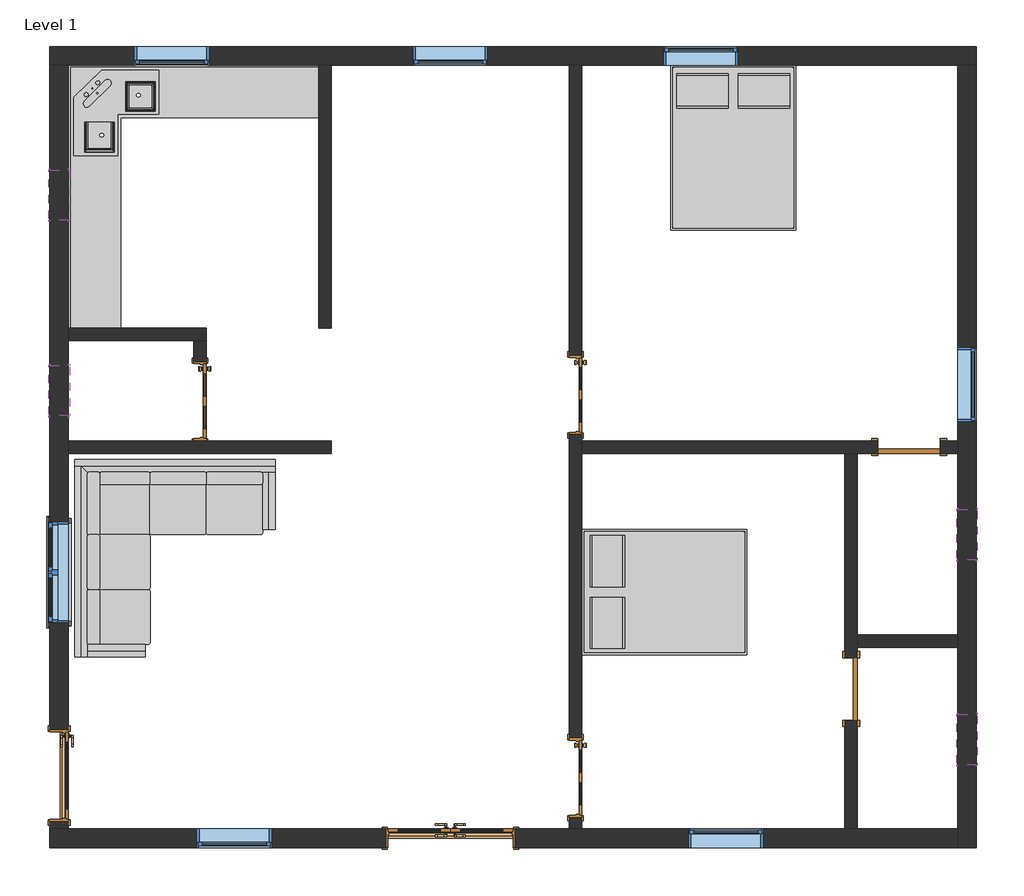
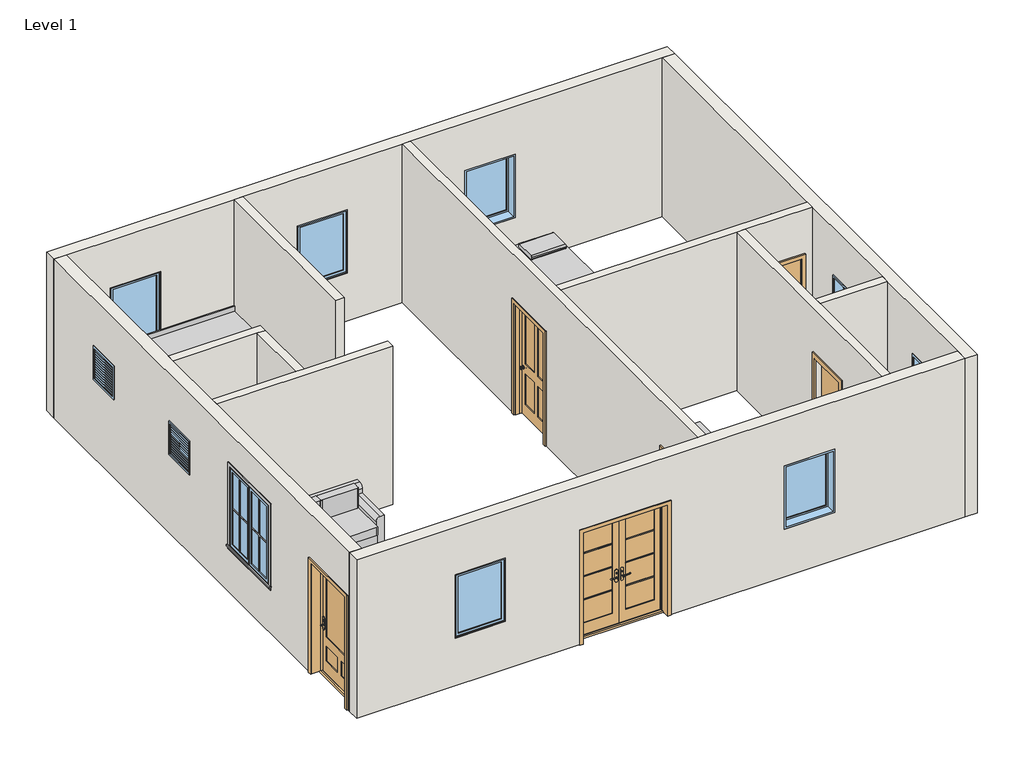
# One storey, incomplete: 12 walls, 11 windows, 7 doors, 4 furniture elements, 4 proxies, 1 flow terminal.
"""IFC4 building model written with IfcOpenShell, lengths in millimetres."""

from ifc_helpers import new_model, si_unit, frame, origin, origin_with_axes, place, context, project, spatial, polyline, outline, extrude, faceted_brep, transform, mapped, element, save
from components import muntin_pattern_2x2_muntin_pattern_2x2_6dad3731, muntin_pattern_2x2_muntin_pattern_2x2_a30a3345, trim_window_exterior_flat_with_sill_92b9b949, trim_window_interior_flat_picture_frame_3bb882cf, door_f44993c8, door_7ffae4ec, door_ecef8289, door_a9addea7, door_e2b13fe9, m_sink_kitchen_corner_1000_x_535mm_64178851, furniture_031_corner_sofa_031_corner_sofa_f2e0ed7f, bed_1_1525_x_2007mm_queen_eef227c3, furniture_c73e3426, window_c1f32544, window_8377141f, window_f2d8fef0, window_407d3824

model = new_model("IFC4")

# Units and contexts
model_context = context("Model", 3, world=origin())
ifc_project = project(units=[si_unit("LENGTHUNIT", "METRE", prefix="MILLI")], contexts=[model_context])

# Site, building, storey
site = spatial("IfcSite", under=ifc_project)
building = spatial("IfcBuilding", under=site)
storey = spatial("IfcBuildingStorey", under=building, Name="Level 1", Elevation=0.0)

# Proxies
placement = place(None, origin())
muntin_pattern_2x2_muntin_pattern_2x2_shape = muntin_pattern_2x2_muntin_pattern_2x2_6dad3731(model_context)
element("IfcBuildingElementProxy", 1, Name="Muntin Pattern_2x2 : Muntin Pattern_2x2", ObjectType="Muntin Pattern_2x2 : Muntin Pattern_2x2", at=placement, inside=storey, context=model_context, shape_type="MappedRepresentation", body=[
    mapped(muntin_pattern_2x2_muntin_pattern_2x2_shape, transform((-13726.9829271, 1900.6806548, 984.25), x_axis=(0.0, 1.0, 0.0), y_axis=(-1.0, 0.0, 0.0), z_axis=(0.0, 0.0, 1.0))),
])
muntin_pattern_2x2_muntin_pattern_2x2_2_shape = muntin_pattern_2x2_muntin_pattern_2x2_a30a3345(model_context)
element("IfcBuildingElementProxy", 2, Name="Muntin Pattern_2x2 : Muntin Pattern_2x2", ObjectType="Muntin Pattern_2x2 : Muntin Pattern_2x2", at=placement, inside=storey, context=model_context, shape_type="MappedRepresentation", body=[
    mapped(muntin_pattern_2x2_muntin_pattern_2x2_2_shape, transform((-13726.9829271, 2507.1056548, 984.25), x_axis=(0.0, -1.0, 0.0), y_axis=(1.0, 0.0, 0.0), z_axis=(0.0, 0.0, 1.0))),
])
trim_window_exterior_flat_with_sill_shape = trim_window_exterior_flat_with_sill_92b9b949(model_context)
element("IfcBuildingElementProxy", 3, Name="Trim-Window-Exterior-Flat : with Sill", ObjectType="Trim-Window-Exterior-Flat : with Sill", at=placement, inside=storey, context=model_context, shape_type="MappedRepresentation", body=[
    mapped(trim_window_exterior_flat_with_sill_shape, transform((-13736.5079271, 2203.8931548, 2438.4), x_axis=(0.0, -1.0, 0.0), y_axis=(0.0, 0.0, 1.0), z_axis=(-1.0, 0.0, 0.0))),
])
trim_window_interior_flat_picture_frame_shape = trim_window_interior_flat_picture_frame_3bb882cf(model_context)
element("IfcBuildingElementProxy", 4, Name="Trim-Window-Interior-Flat : Picture Frame", ObjectType="Trim-Window-Interior-Flat : Picture Frame", at=placement, inside=storey, context=model_context, shape_type="MappedRepresentation", body=[
    mapped(trim_window_interior_flat_picture_frame_shape, transform((-13507.9079271, 2203.8931548, 2438.4), x_axis=(0.0, 1.0, 0.0), y_axis=(0.0, 0.0, 1.0), z_axis=(1.0, 0.0, 0.0))),
])

# Doors
door_shape = door_f44993c8(model_context)
element("IfcDoor", 5, ObjectType="42\" x 84\"", at=placement, inside=storey, context=model_context, shape_type="MappedRepresentation", body=[
    mapped(door_shape, transform((-13619.0329271, -272.6068452, 0.0), x_axis=(0.0, 1.0, 0.0), y_axis=(-1.0, 0.0, 0.0), z_axis=(0.0, 0.0, 1.0))),
])
door_2_shape = door_7ffae4ec(model_context)
element("IfcDoor", 6, ObjectType="Door-Exterior-Double-Full Glass-Wood_Clad : 60\" x 84\"", at=placement, inside=storey, context=model_context, shape_type="MappedRepresentation", body=[
    mapped(door_2_shape, transform((-8859.7079271, -1031.4318452, 0.0), x_axis=(1.0, 0.0, 0.0), y_axis=(0.0, 1.0, 0.0), z_axis=(0.0, 0.0, 1.0))),
])
door_3_shape = door_ecef8289(model_context)
element("IfcDoor", 7, ObjectType="Door-Interior-Single-4_Panel-Wood : 36\" x 84\"", at=placement, inside=storey, context=model_context, shape_type="MappedRepresentation", body=[
    mapped(door_3_shape, transform((-11904.5329271, 4286.6931548, 0.0), x_axis=(0.0, -1.0, 0.0), y_axis=(1.0, 0.0, 0.0), z_axis=(0.0, 0.0, 1.0))),
])
element("IfcDoor", 8, ObjectType="Door-Interior-Single-4_Panel-Wood : 36\" x 84\"", at=placement, inside=storey, context=model_context, shape_type="MappedRepresentation", body=[
    mapped(door_3_shape, transform((-7332.5329271, 4362.8931548, 0.0), x_axis=(0.0, -1.0, 0.0), y_axis=(1.0, 0.0, 0.0), z_axis=(0.0, 0.0, 1.0))),
])
element("IfcDoor", 9, ObjectType="Door-Interior-Single-4_Panel-Wood : 36\" x 84\"", at=placement, inside=storey, context=model_context, shape_type="MappedRepresentation", body=[
    mapped(door_3_shape, transform((-7332.5329271, -298.0068452, 0.0), x_axis=(0.0, -1.0, 0.0), y_axis=(1.0, 0.0, 0.0), z_axis=(0.0, 0.0, 1.0))),
])
door_4_shape = door_a9addea7(model_context)
element("IfcDoor", 10, ObjectType="Single-Flush : 30\" x 84\"", at=placement, inside=storey, context=model_context, shape_type="MappedRepresentation", body=[
    mapped(door_4_shape, transform((-3278.0579271, 3727.8931548, 0.0), x_axis=(-1.0, 0.0, 0.0), y_axis=(0.0, -1.0, 0.0), z_axis=(0.0, 0.0, 1.0))),
])
door_5_shape = door_e2b13fe9(model_context)
element("IfcDoor", 11, ObjectType="Single-Flush : 30\" x 84\"", at=placement, inside=storey, context=model_context, shape_type="MappedRepresentation", body=[
    mapped(door_5_shape, transform((-3982.9079271, 781.4931548, 0.0), x_axis=(0.0, 1.0, 0.0), y_axis=(-1.0, 0.0, 0.0), z_axis=(0.0, 0.0, 1.0))),
])

# Flow terminal
m_sink_kitchen_corner_1000_x_535mm_shape = m_sink_kitchen_corner_1000_x_535mm_64178851(model_context)
element("IfcFlowTerminal", 12, ObjectType="M_Sink Kitchen-Corner : 1000 x 535mm", at=placement, inside=storey, context=model_context, shape_type="MappedRepresentation", body=[
    mapped(m_sink_kitchen_corner_1000_x_535mm_shape, transform((-13040.1393389, 9177.3480874, 14.4), x_axis=(1.0, 0.0, 0.0), y_axis=(0.0, 1.0, 0.0), z_axis=(0.0, 0.0, 1.0))),
])

# Furniture
furniture_031_corner_sofa_031_corner_sofa_shape = furniture_031_corner_sofa_031_corner_sofa_f2e0ed7f(model_context)
element("IfcFurniture", 13, ObjectType="031_corner_sofa : 031_corner_sofa", at=placement, inside=storey, context=model_context, shape_type="MappedRepresentation", body=[
    mapped(furniture_031_corner_sofa_031_corner_sofa_shape, transform((-12212.5079271, 2661.0931548, 0.0), x_axis=(1.0, 0.0, 0.0), y_axis=(0.0, 1.0, 0.0), z_axis=(0.0, 0.0, 1.0))),
])
bed_1_1525_x_2007mm_queen_shape = bed_1_1525_x_2007mm_queen_eef227c3(model_context)
element("IfcFurniture", 14, ObjectType="Bed (1) : 1525 x 2007mm - Queen", at=placement, inside=storey, context=model_context, shape_type="MappedRepresentation", body=[
    mapped(bed_1_1525_x_2007mm_queen_shape, transform((-5757.0603861, 7607.022663, 0.0), x_axis=(1.0, 0.0, 0.0), y_axis=(0.0, 1.0, 0.0), z_axis=(0.0, 0.0, 1.0))),
])
element("IfcFurniture", 15, ObjectType="Bed (1) : 1525 x 2007mm - Queen", at=placement, inside=storey, context=model_context, shape_type="MappedRepresentation", body=[
    mapped(bed_1_1525_x_2007mm_queen_shape, transform((-6490.4374353, 1623.3406958, 0.0), x_axis=(0.0, 1.0, 0.0), y_axis=(-1.0, 0.0, 0.0), z_axis=(0.0, 0.0, 1.0))),
])
furniture_shape = furniture_c73e3426(model_context)
element("IfcFurniture", 16, ObjectType="Counter_Top_-_L_Shaped_w_Corner_Sink : 24\" Depth", at=placement, inside=storey, context=model_context, shape_type="MappedRepresentation", body=[
    mapped(furniture_shape, transform((-12307.445632, 8376.0931548, 0.0), x_axis=(1.0, 0.0, 0.0), y_axis=(0.0, 1.0, 0.0), z_axis=(0.0, 0.0, 1.0))),
])

# Walls
element("IfcWall", 17, ObjectType="Generic - 6\"", at=placement, inside=storey, context=model_context, shape_type="SweptSolid", body=[
    extrude(outline(polyline([(-10459.9079271, 5175.6931548), (-10459.9079271, 8376.0931548), (-10307.5079271, 8376.0931548), (-10307.5079271, 5175.6931548), (-10459.9079271, 5175.6931548)])), origin_with_axes(), (0.0, 0.0, 1.0), 3048.0),
])
element("IfcWall", 18, ObjectType="Generic - 6\"", at=placement, inside=storey, context=model_context, shape_type="Brep", body=[
    faceted_brep([(-7411.9079271, -920.3068452, 3048.0), (-7411.9079271, 8376.0931548, 3048.0), (-7411.9079271, 8376.0931548, 0.0), (-7411.9079271, 4845.4931548, 0.0), (-7411.9079271, 4845.4931548, 2159.0), (-7411.9079271, 3880.2931548, 2159.0), (-7411.9079271, 3880.2931548, 0.0), (-7411.9079271, 184.5931548, 0.0), (-7411.9079271, 184.5931548, 2159.0), (-7411.9079271, -780.6068452, 2159.0), (-7411.9079271, -780.6068452, 0.0), (-7411.9079271, -920.3068452, 0.0), (-7259.5079271, 8376.0931548, 3048.0), (-7259.5079271, 3804.0931548, 3048.0), (-7259.5079271, 3651.6931548, 3048.0), (-7259.5079271, -920.3068452, 3048.0), (-7259.5079271, -920.3068452, 0.0), (-7259.5079271, -780.6068452, 0.0), (-7259.5079271, -780.6068452, 2159.0), (-7259.5079271, 184.5931548, 2159.0), (-7259.5079271, 184.5931548, 0.0), (-7259.5079271, 3651.6931548, 0.0), (-7259.5079271, 3804.0931548, 0.0), (-7259.5079271, 3880.2931548, 0.0), (-7259.5079271, 3880.2931548, 2159.0), (-7259.5079271, 4845.4931548, 2159.0), (-7259.5079271, 4845.4931548, 0.0), (-7259.5079271, 8376.0931548, 0.0)], [[[0, 1, 2, 3, 4, 5, 6, 7, 8, 9, 10, 11]], [[12, 13, 14, 15, 16, 17, 18, 19, 20, 21, 22, 23, 24, 25, 26, 27]], [[2, 27, 26, 3]], [[16, 11, 10, 17]], [[6, 23, 22, 21, 20, 7]], [[1, 0, 15, 14, 13, 12]], [[2, 1, 12, 27]], [[0, 11, 16, 15]], [[5, 24, 23, 6]], [[24, 5, 4, 25]], [[25, 4, 3, 26]], [[9, 18, 17, 10]], [[18, 9, 8, 19]], [[19, 8, 7, 20]]]),
])
element("IfcWall", 19, ObjectType="Generic - 6\"", at=placement, inside=storey, context=model_context, shape_type="Brep", body=[
    faceted_brep([(-13507.9079271, 5023.2931548, 0.0), (-11983.9079271, 5023.2931548, 0.0), (-11831.5079271, 5023.2931548, 0.0), (-11831.5079271, 5023.2931548, 3048.0), (-11983.9079271, 5023.2931548, 3048.0), (-13507.9079271, 5023.2931548, 3048.0), (-13507.9079271, 5175.6931548, 0.0), (-13507.9079271, 5175.6931548, 3048.0), (-11831.5079271, 5175.6931548, 3048.0), (-11831.5079271, 5175.6931548, 0.0)], [[[0, 1, 2, 3, 4, 5]], [[6, 7, 8, 9]], [[2, 1, 0, 6, 9]], [[5, 4, 3, 8, 7]], [[0, 5, 7, 6]], [[3, 2, 9, 8]]]),
])
element("IfcWall", 20, ObjectType="Generic - 6\"", at=placement, inside=storey, context=model_context, shape_type="SweptSolid", body=[
    extrude(outline(polyline([(3804.0931548, 3048.0), (5023.2931548, 3048.0), (5023.2931548, 0.0), (4769.2931548, 0.0), (4769.2931548, 2159.0), (3804.0931548, 2159.0), (3804.0931548, 3048.0)])), frame((-11983.9079271, 0.0, 0.0), z_axis=(1.0, 0.0, 0.0), x_axis=(0.0, 1.0, 0.0)), (0.0, 0.0, 1.0), 152.4),
])
element("IfcWall", 21, ObjectType="Generic - 6\"", at=placement, inside=storey, context=model_context, shape_type="Brep", body=[
    faceted_brep([(-13507.9079271, 3651.6931548, 0.0), (-10307.5079271, 3651.6931548, 0.0), (-10307.5079271, 3651.6931548, 3048.0), (-13507.9079271, 3651.6931548, 3048.0), (-13507.9079271, 3804.0931548, 0.0), (-13507.9079271, 3804.0931548, 3048.0), (-11983.9079271, 3804.0931548, 3048.0), (-11831.5079271, 3804.0931548, 3048.0), (-10307.5079271, 3804.0931548, 3048.0), (-10307.5079271, 3804.0931548, 0.0)], [[[0, 1, 2, 3]], [[4, 5, 6, 7, 8, 9]], [[1, 0, 4, 9]], [[2, 1, 9, 8]], [[3, 2, 8, 7, 6, 5]], [[0, 3, 5, 4]]]),
])
element("IfcWall", 22, ObjectType="Generic - 6\"", at=placement, inside=storey, context=model_context, shape_type="Brep", body=[
    faceted_brep([(-7259.5079271, 3651.6931548, 0.0), (-4059.1079271, 3651.6931548, 0.0), (-3906.7079271, 3651.6931548, 0.0), (-3659.0579271, 3651.6931548, 0.0), (-3659.0579271, 3651.6931548, 2133.6), (-2897.0579271, 3651.6931548, 2133.6), (-2897.0579271, 3651.6931548, 0.0), (-2687.5079271, 3651.6931548, 0.0), (-2687.5079271, 3651.6931548, 3048.0), (-3906.7079271, 3651.6931548, 3048.0), (-4059.1079271, 3651.6931548, 3048.0), (-7259.5079271, 3651.6931548, 3048.0), (-3659.0579271, 3804.0931548, 2133.6), (-3659.0579271, 3804.0931548, 0.0), (-7259.5079271, 3804.0931548, 0.0), (-7259.5079271, 3804.0931548, 3048.0), (-2687.5079271, 3804.0931548, 3048.0), (-2687.5079271, 3804.0931548, 0.0), (-2897.0579271, 3804.0931548, 0.0), (-2897.0579271, 3804.0931548, 2133.6)], [[[0, 1, 2, 3, 4, 5, 6, 7, 8, 9, 10, 11]], [[12, 13, 14, 15, 16, 17, 18, 19]], [[18, 17, 7, 6]], [[14, 13, 3, 2, 1, 0]], [[11, 10, 9, 8, 16, 15]], [[8, 7, 17, 16]], [[0, 11, 15, 14]], [[4, 3, 13, 12]], [[5, 4, 12, 19]], [[6, 5, 19, 18]]]),
])
element("IfcWall", 23, ObjectType="Generic - 6\"", at=placement, inside=storey, context=model_context, shape_type="Brep", body=[
    faceted_brep([(-4059.1079271, 3651.6931548, 0.0), (-4059.1079271, 1162.4931548, 0.0), (-4059.1079271, 1162.4931548, 2133.6), (-4059.1079271, 400.4931548, 2133.6), (-4059.1079271, 400.4931548, 0.0), (-4059.1079271, -920.3068452, 0.0), (-4059.1079271, -920.3068452, 3048.0), (-4059.1079271, 3651.6931548, 3048.0), (-3906.7079271, 1162.4931548, 2133.6), (-3906.7079271, 1162.4931548, 0.0), (-3906.7079271, 1289.4931548, 0.0), (-3906.7079271, 1441.8931548, 0.0), (-3906.7079271, 3651.6931548, 0.0), (-3906.7079271, 3651.6931548, 3048.0), (-3906.7079271, 1441.8931548, 3048.0), (-3906.7079271, 1289.4931548, 3048.0), (-3906.7079271, -920.3068452, 3048.0), (-3906.7079271, -920.3068452, 0.0), (-3906.7079271, 400.4931548, 0.0), (-3906.7079271, 400.4931548, 2133.6)], [[[0, 1, 2, 3, 4, 5, 6, 7]], [[8, 9, 10, 11, 12, 13, 14, 15, 16, 17, 18, 19]], [[18, 17, 5, 4]], [[12, 11, 10, 9, 1, 0]], [[7, 6, 16, 15, 14, 13]], [[6, 5, 17, 16]], [[0, 7, 13, 12]], [[2, 1, 9, 8]], [[3, 2, 8, 19]], [[4, 3, 19, 18]]]),
])
element("IfcWall", 24, ObjectType="Generic - 6\"", at=placement, inside=storey, context=model_context, shape_type="SweptSolid", body=[
    extrude(outline(polyline([(-3906.7079271, 1441.8931548), (-2687.5079271, 1441.8931548), (-2687.5079271, 1289.4931548), (-3906.7079271, 1289.4931548), (-3906.7079271, 1441.8931548)])), origin_with_axes(), (0.0, 0.0, 1.0), 3048.0),
])
element("IfcWall", 25, ObjectType="Generic - 9\"", at=placement, inside=storey, context=model_context, shape_type="Brep", body=[
    faceted_brep([(-13736.5079271, 8376.0931548, 0.0), (-13507.9079271, 8376.0931548, 0.0), (-10459.9079271, 8376.0931548, 0.0), (-10307.5079271, 8376.0931548, 0.0), (-7411.9079271, 8376.0931548, 0.0), (-7259.5079271, 8376.0931548, 0.0), (-2687.5079271, 8376.0931548, 0.0), (-2458.9079271, 8376.0931548, 0.0), (-2458.9079271, 8376.0931548, 3048.0), (-2687.5079271, 8376.0931548, 3048.0), (-7259.5079271, 8376.0931548, 3048.0), (-7411.9079271, 8376.0931548, 3048.0), (-10307.5079271, 8376.0931548, 3048.0), (-10459.9079271, 8376.0931548, 3048.0), (-13507.9079271, 8376.0931548, 3048.0), (-13736.5079271, 8376.0931548, 3048.0), (-5354.5079271, 8376.0931548, 2133.6), (-5354.5079271, 8376.0931548, 914.4), (-6268.9079271, 8376.0931548, 914.4), (-6268.9079271, 8376.0931548, 2133.6), (-9316.9079271, 8376.0931548, 2133.6), (-8402.5079271, 8376.0931548, 2133.6), (-8402.5079271, 8376.0931548, 914.4), (-9316.9079271, 8376.0931548, 914.4), (-12707.8079271, 8376.0931548, 2133.6), (-11793.4079271, 8376.0931548, 2133.6), (-11793.4079271, 8376.0931548, 914.4), (-12707.8079271, 8376.0931548, 914.4), (-13736.5079271, 8604.6931548, 0.0), (-13736.5079271, 8604.6931548, 3048.0), (-2458.9079271, 8604.6931548, 3048.0), (-2458.9079271, 8604.6931548, 0.0), (-5354.5079271, 8604.6931548, 2133.6), (-6268.9079271, 8604.6931548, 2133.6), (-6268.9079271, 8604.6931548, 914.4), (-5354.5079271, 8604.6931548, 914.4), (-9316.9079271, 8604.6931548, 2133.6), (-9316.9079271, 8604.6931548, 914.4), (-8402.5079271, 8604.6931548, 914.4), (-8402.5079271, 8604.6931548, 2133.6), (-12707.8079271, 8604.6931548, 2133.6), (-12707.8079271, 8604.6931548, 914.4), (-11793.4079271, 8604.6931548, 914.4), (-11793.4079271, 8604.6931548, 2133.6)], [[[0, 1, 2, 3, 4, 5, 6, 7, 8, 9, 10, 11, 12, 13, 14, 15], [16, 17, 18, 19], [20, 21, 22, 23], [24, 25, 26, 27]], [[28, 29, 30, 31], [32, 33, 34, 35], [36, 37, 38, 39], [40, 41, 42, 43]], [[7, 6, 5, 4, 3, 2, 1, 0, 28, 31]], [[15, 14, 13, 12, 11, 10, 9, 8, 30, 29]], [[8, 7, 31, 30]], [[0, 15, 29, 28]], [[17, 16, 32, 35]], [[18, 17, 35, 34]], [[19, 18, 34, 33]], [[16, 19, 33, 32]], [[37, 36, 20, 23]], [[38, 37, 23, 22]], [[39, 38, 22, 21]], [[36, 39, 21, 20]], [[41, 40, 24, 27]], [[42, 41, 27, 26]], [[43, 42, 26, 25]], [[40, 43, 25, 24]]]),
])
element("IfcWall", 26, ObjectType="Generic - 9\"", at=placement, inside=storey, context=model_context, shape_type="Brep", body=[
    faceted_brep([(-2687.5079271, 8376.0931548, 0.0), (-2687.5079271, 3804.0931548, 0.0), (-2687.5079271, 3651.6931548, 0.0), (-2687.5079271, 1441.8931548, 0.0), (-2687.5079271, 1289.4931548, 0.0), (-2687.5079271, -920.3068452, 0.0), (-2687.5079271, -1148.9068452, 0.0), (-2687.5079271, -1148.9068452, 3048.0), (-2687.5079271, -920.3068452, 3048.0), (-2687.5079271, 1289.4931548, 3048.0), (-2687.5079271, 1441.8931548, 3048.0), (-2687.5079271, 3651.6931548, 3048.0), (-2687.5079271, 3804.0931548, 3048.0), (-2687.5079271, 8376.0931548, 3048.0), (-2687.5079271, 4032.6931548, 2133.6), (-2687.5079271, 4032.6931548, 914.4), (-2687.5079271, 4947.0931548, 914.4), (-2687.5079271, 4947.0931548, 2133.6), (-2687.5079271, 2356.2931548, 2133.6), (-2687.5079271, 2356.2931548, 1524.0), (-2687.5079271, 2965.8931548, 1524.0), (-2687.5079271, 2965.8931548, 2133.6), (-2687.5079271, -139.2568452, 2133.6), (-2687.5079271, -139.2568452, 1524.0), (-2687.5079271, 470.3431548, 1524.0), (-2687.5079271, 470.3431548, 2133.6), (-2458.9079271, 8376.0931548, 0.0), (-2458.9079271, 8376.0931548, 3048.0), (-2458.9079271, -1148.9068452, 3048.0), (-2458.9079271, -1148.9068452, 0.0), (-2458.9079271, 4032.6931548, 2133.6), (-2458.9079271, 4947.0931548, 2133.6), (-2458.9079271, 4947.0931548, 914.4), (-2458.9079271, 4032.6931548, 914.4), (-2458.9079271, 2356.2931548, 2133.6), (-2458.9079271, 2965.8931548, 2133.6), (-2458.9079271, 2965.8931548, 1524.0), (-2458.9079271, 2356.2931548, 1524.0), (-2458.9079271, -139.2568452, 2133.6), (-2458.9079271, 470.3431548, 2133.6), (-2458.9079271, 470.3431548, 1524.0), (-2458.9079271, -139.2568452, 1524.0)], [[[0, 1, 2, 3, 4, 5, 6, 7, 8, 9, 10, 11, 12, 13], [14, 15, 16, 17], [18, 19, 20, 21], [22, 23, 24, 25]], [[26, 27, 28, 29], [30, 31, 32, 33], [34, 35, 36, 37], [38, 39, 40, 41]], [[6, 5, 4, 3, 2, 1, 0, 26, 29]], [[13, 12, 11, 10, 9, 8, 7, 28, 27]], [[0, 13, 27, 26]], [[7, 6, 29, 28]], [[15, 14, 30, 33]], [[16, 15, 33, 32]], [[17, 16, 32, 31]], [[14, 17, 31, 30]], [[19, 18, 34, 37]], [[20, 19, 37, 36]], [[21, 20, 36, 35]], [[18, 21, 35, 34]], [[23, 22, 38, 41]], [[24, 23, 41, 40]], [[25, 24, 40, 39]], [[22, 25, 39, 38]]]),
])
element("IfcWall", 27, ObjectType="Generic - 9\"", at=placement, inside=storey, context=model_context, shape_type="Brep", body=[
    faceted_brep([(-13736.5079271, -920.3068452, 3048.0), (-13507.9079271, -920.3068452, 3048.0), (-7411.9079271, -920.3068452, 3048.0), (-7259.5079271, -920.3068452, 3048.0), (-4059.1079271, -920.3068452, 3048.0), (-3906.7079271, -920.3068452, 3048.0), (-2687.5079271, -920.3068452, 3048.0), (-2687.5079271, -920.3068452, 0.0), (-3906.7079271, -920.3068452, 0.0), (-4059.1079271, -920.3068452, 0.0), (-7259.5079271, -920.3068452, 0.0), (-7411.9079271, -920.3068452, 0.0), (-8072.3079271, -920.3068452, 0.0), (-8072.3079271, -920.3068452, 2159.0), (-9647.1079271, -920.3068452, 2159.0), (-9647.1079271, -920.3068452, 0.0), (-13507.9079271, -920.3068452, 0.0), (-13736.5079271, -920.3068452, 0.0), (-11945.8079271, -920.3068452, 2133.6), (-11945.8079271, -920.3068452, 914.4), (-11031.4079271, -920.3068452, 914.4), (-11031.4079271, -920.3068452, 2133.6), (-5049.7079271, -920.3068452, 2133.6), (-5964.1079271, -920.3068452, 2133.6), (-5964.1079271, -920.3068452, 914.4), (-5049.7079271, -920.3068452, 914.4), (-2687.5079271, -1148.9068452, 3048.0), (-13736.5079271, -1148.9068452, 3048.0), (-13736.5079271, -1148.9068452, 0.0), (-9647.1079271, -1148.9068452, 0.0), (-9647.1079271, -1148.9068452, 2159.0), (-8072.3079271, -1148.9068452, 2159.0), (-8072.3079271, -1148.9068452, 0.0), (-2687.5079271, -1148.9068452, 0.0), (-11945.8079271, -1148.9068452, 2133.6), (-11031.4079271, -1148.9068452, 2133.6), (-11031.4079271, -1148.9068452, 914.4), (-11945.8079271, -1148.9068452, 914.4), (-5049.7079271, -1148.9068452, 2133.6), (-5049.7079271, -1148.9068452, 914.4), (-5964.1079271, -1148.9068452, 914.4), (-5964.1079271, -1148.9068452, 2133.6)], [[[0, 1, 2, 3, 4, 5, 6, 7, 8, 9, 10, 11, 12, 13, 14, 15, 16, 17], [18, 19, 20, 21], [22, 23, 24, 25]], [[26, 27, 28, 29, 30, 31, 32, 33], [34, 35, 36, 37], [38, 39, 40, 41]], [[7, 33, 32, 12, 11, 10, 9, 8]], [[28, 17, 16, 15, 29]], [[6, 5, 4, 3, 2, 1, 0, 27, 26]], [[7, 6, 26, 33]], [[0, 17, 28, 27]], [[31, 13, 12, 32]], [[13, 31, 30, 14]], [[14, 30, 29, 15]], [[19, 18, 34, 37]], [[20, 19, 37, 36]], [[21, 20, 36, 35]], [[18, 21, 35, 34]], [[39, 38, 22, 25]], [[40, 39, 25, 24]], [[41, 40, 24, 23]], [[38, 41, 23, 22]]]),
])
element("IfcWall", 28, ObjectType="Generic - 9\"", at=placement, inside=storey, context=model_context, shape_type="Brep", body=[
    faceted_brep([(-13507.9079271, 8376.0931548, 3048.0), (-13507.9079271, 5175.6931548, 3048.0), (-13507.9079271, 5023.2931548, 3048.0), (-13507.9079271, 3804.0931548, 3048.0), (-13507.9079271, 3651.6931548, 3048.0), (-13507.9079271, -920.3068452, 3048.0), (-13507.9079271, -920.3068452, 0.0), (-13507.9079271, -831.4068452, 0.0), (-13507.9079271, -831.4068452, 2159.0), (-13507.9079271, 286.1931548, 2159.0), (-13507.9079271, 286.1931548, 0.0), (-13507.9079271, 3651.6931548, 0.0), (-13507.9079271, 3804.0931548, 0.0), (-13507.9079271, 5023.2931548, 0.0), (-13507.9079271, 5175.6931548, 0.0), (-13507.9079271, 8376.0931548, 0.0), (-13507.9079271, 2813.4931548, 2438.4), (-13507.9079271, 2813.4931548, 914.4), (-13507.9079271, 1594.2931548, 914.4), (-13507.9079271, 1594.2931548, 2438.4), (-13507.9079271, 6490.1431548, 2133.6), (-13507.9079271, 7099.7431548, 2133.6), (-13507.9079271, 7099.7431548, 1524.0), (-13507.9079271, 6490.1431548, 1524.0), (-13507.9079271, 4108.8931548, 2133.6), (-13507.9079271, 4718.4931548, 2133.6), (-13507.9079271, 4718.4931548, 1524.0), (-13507.9079271, 4108.8931548, 1524.0), (-13736.5079271, -920.3068452, 3048.0), (-13736.5079271, 8376.0931548, 3048.0), (-13736.5079271, 8376.0931548, 0.0), (-13736.5079271, 286.1931548, 0.0), (-13736.5079271, 286.1931548, 2159.0), (-13736.5079271, -831.4068452, 2159.0), (-13736.5079271, -831.4068452, 0.0), (-13736.5079271, -920.3068452, 0.0), (-13736.5079271, 2813.4931548, 2438.4), (-13736.5079271, 1594.2931548, 2438.4), (-13736.5079271, 1594.2931548, 914.4), (-13736.5079271, 2813.4931548, 914.4), (-13736.5079271, 6490.1431548, 2133.6), (-13736.5079271, 6490.1431548, 1524.0), (-13736.5079271, 7099.7431548, 1524.0), (-13736.5079271, 7099.7431548, 2133.6), (-13736.5079271, 4108.8931548, 2133.6), (-13736.5079271, 4108.8931548, 1524.0), (-13736.5079271, 4718.4931548, 1524.0), (-13736.5079271, 4718.4931548, 2133.6)], [[[0, 1, 2, 3, 4, 5, 6, 7, 8, 9, 10, 11, 12, 13, 14, 15], [16, 17, 18, 19], [20, 21, 22, 23], [24, 25, 26, 27]], [[28, 29, 30, 31, 32, 33, 34, 35], [36, 37, 38, 39], [40, 41, 42, 43], [44, 45, 46, 47]], [[6, 35, 34, 7]], [[30, 15, 14, 13, 12, 11, 10, 31]], [[5, 4, 3, 2, 1, 0, 29, 28]], [[0, 15, 30, 29]], [[6, 5, 28, 35]], [[9, 32, 31, 10]], [[32, 9, 8, 33]], [[33, 8, 7, 34]], [[17, 16, 36, 39]], [[18, 17, 39, 38]], [[19, 18, 38, 37]], [[16, 19, 37, 36]], [[41, 40, 20, 23]], [[42, 41, 23, 22]], [[43, 42, 22, 21]], [[40, 43, 21, 20]], [[45, 44, 24, 27]], [[46, 45, 27, 26]], [[47, 46, 26, 25]], [[44, 47, 25, 24]]]),
])

# Windows
window_shape = window_c1f32544(model_context)
element("IfcWindow", 29, ObjectType="Fixed : 36\" x 48\"", at=placement, inside=storey, context=model_context, shape_type="MappedRepresentation", body=[
    mapped(window_shape, transform((-11526.7079271, -1034.6068452, 0.0), x_axis=(-1.0, 0.0, 0.0), y_axis=(0.0, -1.0, 0.0), z_axis=(0.0, 0.0, 1.0))),
])
element("IfcWindow", 30, ObjectType="Fixed : 36\" x 48\"", at=placement, inside=storey, context=model_context, shape_type="MappedRepresentation", body=[
    mapped(window_shape, transform((-5468.8079271, -1034.6068452, 0.0), x_axis=(1.0, 0.0, 0.0), y_axis=(0.0, 1.0, 0.0), z_axis=(0.0, 0.0, 1.0))),
])
element("IfcWindow", 31, ObjectType="Fixed : 36\" x 48\"", at=placement, inside=storey, context=model_context, shape_type="MappedRepresentation", body=[
    mapped(window_shape, transform((-2573.2079271, 4451.7931548, 0.0), x_axis=(0.0, -1.0, 0.0), y_axis=(1.0, 0.0, 0.0), z_axis=(0.0, 0.0, 1.0))),
])
element("IfcWindow", 32, ObjectType="Fixed : 36\" x 48\"", at=placement, inside=storey, context=model_context, shape_type="MappedRepresentation", body=[
    mapped(window_shape, transform((-5773.6079271, 8490.3931548, 0.0), x_axis=(1.0, 0.0, 0.0), y_axis=(0.0, 1.0, 0.0), z_axis=(0.0, 0.0, 1.0))),
])
element("IfcWindow", 33, ObjectType="Fixed : 36\" x 48\"", at=placement, inside=storey, context=model_context, shape_type="MappedRepresentation", body=[
    mapped(window_shape, transform((-8897.8079271, 8490.3931548, 0.0), x_axis=(-1.0, 0.0, 0.0), y_axis=(0.0, -1.0, 0.0), z_axis=(0.0, 0.0, 1.0))),
])
element("IfcWindow", 34, ObjectType="Fixed : 36\" x 48\"", at=placement, inside=storey, context=model_context, shape_type="MappedRepresentation", body=[
    mapped(window_shape, transform((-12288.7079271, 8490.3931548, 0.0), x_axis=(-1.0, 0.0, 0.0), y_axis=(0.0, -1.0, 0.0), z_axis=(0.0, 0.0, 1.0))),
])
window_2_shape = window_8377141f(model_context)
element("IfcWindow", 35, ObjectType="Window-Casement-Double : 48\" x 60\"", at=placement, inside=storey, context=model_context, shape_type="MappedRepresentation", body=[
    mapped(window_2_shape, transform((-13622.2079271, 2203.8931548, 0.0), x_axis=(0.0, 1.0, 0.0), y_axis=(-1.0, 0.0, 0.0), z_axis=(0.0, 0.0, 1.0))),
])
window_3_shape = window_f2d8fef0(model_context)
element("IfcWindow", 36, ObjectType="Window-Louvers : 24\" x 24\"", at=placement, inside=storey, context=model_context, shape_type="MappedRepresentation", body=[
    mapped(window_3_shape, transform((-13628.5579271, 6794.9431548, 609.6), x_axis=(0.0, 1.0, 0.0), y_axis=(-1.0, 0.0, 0.0), z_axis=(0.0, 0.0, 1.0))),
])
element("IfcWindow", 37, ObjectType="Window-Louvers : 24\" x 24\"", at=placement, inside=storey, context=model_context, shape_type="MappedRepresentation", body=[
    mapped(window_3_shape, transform((-13628.5579271, 4413.6931548, 609.6), x_axis=(0.0, 1.0, 0.0), y_axis=(-1.0, 0.0, 0.0), z_axis=(0.0, 0.0, 1.0))),
])
window_4_shape = window_407d3824(model_context)
element("IfcWindow", 38, ObjectType="Window-Louvers : 24\" x 24\"", at=placement, inside=storey, context=model_context, shape_type="MappedRepresentation", body=[
    mapped(window_4_shape, transform((-2566.8579271, 2661.0931548, 609.6), x_axis=(0.0, 1.0, 0.0), y_axis=(-1.0, 0.0, 0.0), z_axis=(0.0, 0.0, 1.0))),
])
element("IfcWindow", 39, ObjectType="Window-Louvers : 24\" x 24\"", at=placement, inside=storey, context=model_context, shape_type="MappedRepresentation", body=[
    mapped(window_4_shape, transform((-2566.8579271, 165.5431548, 609.6), x_axis=(0.0, 1.0, 0.0), y_axis=(-1.0, 0.0, 0.0), z_axis=(0.0, 0.0, 1.0))),
])

save(model, "model.ifc")

# Revit data of these elements
# Type "Muntin Pattern_2x2 : Muntin Pattern_2x2"
#   Width [instance default] = 4' - 0"
#   Thickness = 0' - 0 1/2"
#   Height [instance default] = 4' - 0"
#   Distance = 0' - 0 3/4"
#   Interior Material [instance default] = none
#   Exterior Material [instance default] = none
#   Default Elevation = 0
# Type "Trim-Window-Exterior-Flat : with Sill"
#   Trim Width = 0' - 2 1/4"
#   Trim Thickness_Picture Frame = 0' - 1 1/4"
#   Trim Thickness_with Sill = 0' - 0 3/4"
#   Sill Thickness = 0' - 1 1/4"
#   Opening Width [instance default] = 2' - 0"
#   Opening Height [instance default] = 3' - 0"
#   Default Elevation = 4' - 0"
#   Sill = yes
#   Picture Frame = no
#   Trim Material [instance default] = none
# Type "Trim-Window-Interior-Flat : Picture Frame"
#   Trim Thickness_Picture Frame = 0' - 1 1/4"
#   Trim Width = 0' - 2 1/4"
#   Trim Thickness_with Sill = 0' - 0 3/4"
#   Sill Thickness = 0' - 1 1/4"
#   Opening Width [instance default] = 2' - 0"
#   Opening Height [instance default] = 3' - 0"
#   Default Elevation = 4' - 0"
#   Sill = no
#   Picture Frame = yes
#   Trim Material [instance default] = none
# Type "42\" x 84\""
#   Type Mark = "11"
#   Assembly Code = "B2030100"
#   Analytic Construction = "French door, wood frame with single glass"
#   Threshold Offset [instance default] = 0' - 0 1/2"
#   Thickness = 0' - 1 3/8"
#   Thermal Resistance (R) = 1.0696 (h·ft²·°F)/BTU
#   Swing Angle [instance default] = 90.00°
#   Stiles = 0' - 4 3/4"
#   Rough Width = 3' - 8"
#   Rough Height = 7' - 1"
#   Radius = 2' - 4 29/32"
#   Lock Rail = 0' - 7 1/8"
#   Height = 7' - 0"
#   Width = 3' - 6"
#   Heat Transfer Coefficient (U) = 0.9350 BTU/(h·ft²·°F)
#   Door Offset [instance default] = 0' - 0"
#   Bottom Rail = 0' - 9 1/2"
#   Threshold [instance default] = yes
#   Function = 1
#   Exterior Trim [instance default] = yes
#   Trim Material = Cherry
#   Threshold Material = Cherry
#   Panel Material = Cherry
#   Glazing = Glass
#   Frame Material = Cherry
#   Door Handle Material = Aluminum
#   Visual Light Transmittance = 0
#   Solar Heat Gain Coefficient = 0
#   Wall Closure = (empty or 0)
#   Construction Type = (empty or 0)
# Type "Door-Exterior-Double-Full Glass-Wood_Clad : 60\" x 84\""
#   Type Mark = "12"
#   Assembly Code = "B2030100"
#   Analytic Construction = "French door, wood frame with double glass"
#   Top Rail = 0' - 4 11/16"
#   Threshold Offset [instance default] = 0' - 0 1/2"
#   Thickness = 0' - 1 3/8"
#   Thermal Resistance (R) = 1.9158 (h·ft²·°F)/BTU
#   Swing Angle [instance default] = 90.00°
#   Stiles = 0' - 4 3/4"
#   Rough Width = 5' - 2"
#   Rough Height = 7' - 1"
#   Panel Width = 2' - 6"
#   Door Offset [instance default] = 0' - 0"
#   Height = 7' - 0"
#   Width = 5' - 0"
#   Heat Transfer Coefficient (U) = 0.5220 BTU/(h·ft²·°F)
#   Bottom Rail = 0' - 9 1/8"
#   Exterior Trim [instance default] = yes
#   Threshold [instance default] = yes
#   Show Grill [instance default] = yes
#   Function = 1
#   Trim Material = Cherry
#   Threshold Material = Cherry
#   Panel Material = Cherry
#   Glazing = Glass
#   Frame Material = Cherry
#   Door Handle Material = Aluminum
#   Visual Light Transmittance = 0
#   Solar Heat Gain Coefficient = 0
#   Wall Closure = (empty or 0)
#   Construction Type = (empty or 0)
# Type "Door-Interior-Single-4_Panel-Wood : 36\" x 84\""
#   Type Mark = "8"
#   Assembly Code = "C1020300"
#   Analytic Construction = "Wooden"
#   Top Rail = 0' - 4 11/16"
#   Thickness = 0' - 1 3/8"
#   Thermal Resistance (R) = 2.5876 (h·ft²·°F)/BTU
#   Swing Angle [instance default] = 90.00°
#   Stiles = 0' - 4 3/4"
#   Rough Width = 3' - 2"
#   Rough Height = 7' - 1"
#   Mullion = 0' - 4 1/2"
#   Lock Rail = 0' - 7 1/2"
#   Height = 7' - 0"
#   Width = 3' - 0"
#   Heat Transfer Coefficient (U) = 0.3865 BTU/(h·ft²·°F)
#   Bottom Rail = 0' - 9 1/8"
#   Trim Material = Cherry
#   Panel Material = Cherry
#   Frame Material = Cherry
#   Door Handle Material = Aluminum
#   Visual Light Transmittance = 0
#   Solar Heat Gain Coefficient = 0
#   Wall Closure = (empty or 0)
#   Function = (empty or 0)
# Type "Single-Flush : 30\" x 84\""
#   Type Mark = "4"
#   Construction Type Id = "MDOOR"
#   Assembly Code = "C1020"
#   Analytic Construction = "Metal"
#   Thickness = 0' - 2"
#   Heat Transfer Coefficient (U) = 0.651978 BTU/(h·ft²·°F)
#   Height = 7' - 0"
#   Trim Projection Ext = 0' - 1"
#   Trim Projection Int = 0' - 1"
#   Trim Width = 0' - 3"
#   Width = 2' - 6"
#   Define Thermal Properties by = 1
#   Define Thermal Properties by = 1
#   Door Material = Door - Panel
#   Frame Material = Door - Frame
#   Visual Light Transmittance = 0
#   Solar Heat Gain Coefficient = 0
#   Function = (empty or 0)
#   Wall Closure = (empty or 0)
# Type "M_Sink Kitchen-Corner : 1000 x 535mm"
#   Sink Offset (Side) [instance default] = 0' - 1.62205"
#   Sink Offset (Front) = 0' - 1 1/2"
#   Sink Length [instance default] = 1' - 4.56299"
#   Counter Height [instance default] = 2' - 11.43307"
#   Depth = 1' - 9.06299"
#   Width = 1' - 9.06299"
#   Fixture Material = Metal - Steel, Polished
#   Sink Material = Metal - Steel, Polished
#   Default Elevation = 0
#   Assembly Code = ""
# Type "031_corner_sofa : 031_corner_sofa"
#   Default Elevation = 0
# Type "Bed (1) : 1525 x 2007mm - Queen"
#   Keynote = "N"
#   Length = 6' - 7.01575"
#   Width = 5' - 0.03937"
#   Material Frame = Wood - Birch
#   Material Mattress = Textile - White
#   Default Elevation = 0
# Type "Counter_Top_-_L_Shaped_w_Corner_Sink : 24\" Depth"
#   Assembly Code = "C1030400"
#   Sink Opening [instance default] = 1' - 4.56299"
#   Sink Offset (Front) [instance default] = 0' - 2.98406"
#   Counter Thickness = 0' - 1 1/2"
#   Depth = 2' - 1"
#   Height = 3' - 0"
#   Length - Leg 1 [instance default] = 8' - 0"
#   Length - Leg 2 [instance default] = 6' - 0"
#   Counter Top Material = none
#   Default Elevation = 0
# Type "Generic - 6\""
#   Assembly Code = "B2010"
#   Layers, outside or top first: 0' - 6" no material (function 1)
# Type "Generic - 9\""
#   Assembly Code = "B2010"
#   Layers, outside or top first: 0' - 9" no material (function 1)
# Type "Fixed : 36\" x 48\""
#   Type Mark = "1"
#   Construction Type Id = "GSP4R"
#   Assembly Code = "B2020100"
#   Analytic Construction = "1/8 in Pilkington single glazing"
#   Visual Light Transmittance = 0.9
#   Solar Heat Gain Coefficient = 0.78
#   Heat Transfer Coefficient (U) = 0.6496 BTU/(h·ft²·°F)
#   Height = 4' - 0"
#   Default Sill Height = 3' - 0"
#   Width = 3' - 0"
#   Window Inset = 0' - 0 3/4"
#   Define Thermal Properties by = 1
#   Define Thermal Properties by = 1
#   Glass Pane Material = Glass
#   Sash Material = Sash
#   Wall Closure = (empty or 0)
# Type "Window-Casement-Double : 48\" x 60\""
#   Type Mark = "16"
#   Fire Rating = "0.5h"
#   Assembly Code = "B2020100"
#   Analytic Construction = "Double glazing - domestic"
#   Frame Extension [instance default] = 0' - 0 1/4"
#   Window Inset [instance default] = 0' - 0"
#   Wall Thickness [instance default] = 0' - 6"
#   Interior Wall Closure [instance default] = 0' - 2 1/4"
#   Half Width = 2' - 0"
#   Visual Light Transmittance = 0.81
#   Thermal Resistance (R) = 1.8146 (h·ft²·°F)/BTU
#   Solar Heat Gain Coefficient = 0.76
#   Rough Width = 4' - 0 1/2"
#   Rough Height = 5' - 0 1/2"
#   Height = 5' - 0"
#   Heat Transfer Coefficient (U) = 0.5511 BTU/(h·ft²·°F)
#   Exterior Wall Closure [instance default] = 0' - 1 1/4"
#   Extension Jamb [instance default] = 0' - 2 1/4"
#   Default Sill Height = 3' - 0"
#   Width = 4' - 0"
#   Define Thermal Properties by = 0
#   Muntin Visibility = yes
#   Interior Trim Visibility [instance default] = yes
#   Exterior Trim Visibility [instance default] = yes
#   Extension Jamb Visibility [instance default] = yes
#   Interior Trim Material = Wood - Stained
#   Muntin Pattern = Muntin Pattern_2x2 : Muntin Pattern_2x2
#   Interior Trim = Trim-Window-Interior-Flat : Picture Frame
#   Interior Frame Material = Wood - Stained
#   Glass Panel Material = Glass
#   Exterior Trim Material = Clad - White
#   Exterior Trim = Trim-Window-Exterior-Flat : with Sill
#   Exterior Frame Material = Clad - White
#   Wall Closure = (empty or 0)
# Type "Window-Louvers : 24\" x 24\""
#   Type Mark = "18"
#   Construction Type Id = "GSP4R"
#   Assembly Code = "B20"
#   Analytic Construction = "1/8 in Pilkington single glazing"
#   Visual Light Transmittance = 0.9
#   Thermal Resistance (R) = 1.53941 (h·ft²·°F)/BTU
#   Solar Heat Gain Coefficient = 0.78
#   Max Height = 1' - 11.74264"
#   Height = 2' - 0"
#   Heat Transfer Coefficient (U) = 0.6496 BTU/(h·ft²·°F)
#   Blade Width [instance default] = 1' - 10 1/2"
#   Blade Vertical Thickness = 0' - 0.35355"
#   Blade Thickness = 0' - 0 1/4"
#   Blade Spacing = 0' - 1 1/2"
#   Blade Height = 0' - 1.85355"
#   Blade Depth = 0' - 3"
#   Blade Angle = 45.00°
#   Default Sill Height = 3' - 0"
#   Trim Projection_Exterior = 0' - 0 1/2"
#   Trim Projection_Interior = 0' - 0 1/2"
#   Trim Width_Exterior = 0' - 1 1/2"
#   Trim Width_Interior = 0' - 1 1/2"
#   Width = 2' - 0"
#   Max Blade Count = 12
#   Define Thermal Properties by = 1
#   Blade Count = 12
#   Frame Material = Birch
#   Louver Material = Birch
#   Trim Exterior Material = Birch
#   Trim Interior Material = Birch
#   Wall Closure = (empty or 0)
# Elements 1, 2 (IfcBuildingElementProxy, "Muntin Pattern_2x2 : Muntin Pattern_2x2")
#   Width = 1' - 6 5/8"
#   Height = 4' - 6 1/2"
#   Interior Material = Wood - Stained
#   Exterior Material = Clad - White
#   Phase Created = New Construction
#   Materials on its faces: "Clad - White", "Wood - Stained"
# Element 3 (IfcBuildingElementProxy, "Trim-Window-Exterior-Flat : with Sill")
#   Opening Width = 4' - 0"
#   Opening Height = 5' - 0"
#   Trim Material = Clad - White
#   Phase Created = New Construction
#   Materials on its faces: "Clad - White"
# Element 4 (IfcBuildingElementProxy, "Trim-Window-Interior-Flat : Picture Frame")
#   Opening Width = 4' - 0"
#   Opening Height = 5' - 0"
#   Trim Material = Wood - Stained
#   Phase Created = New Construction
#   Materials on its faces: "Wood - Stained"
# Element 5 (IfcDoor, "42\" x 84\"")
#   Threshold Offset = 0' - 0 1/2"
#   Swing Angle = 90.00°
#   Door Offset = 0' - 0"
#   Threshold = yes
#   Exterior Trim = yes
#   Phase Created = New Construction
#   Materials on its faces: "Cherry", "Aluminum", "Glass"
# Element 6 (IfcDoor, "Door-Exterior-Double-Full Glass-Wood_Clad : 60\" x 84\"")
#   Threshold Offset = 0' - 0 1/2"
#   Swing Angle = 90.00°
#   Door Offset = 0' - 0"
#   Threshold = yes
#   Show Grill = yes
#   Exterior Trim = yes
#   Phase Created = New Construction
#   Materials on its faces: "Cherry", "Aluminum", "Glass"
# Elements 7, 8, 9 (IfcDoor, "Door-Interior-Single-4_Panel-Wood : 36\" x 84\"")
#   Swing Angle = 90.00°
#   Phase Created = New Construction
#   Materials on its faces: "Cherry", "Aluminum"
# Elements 10, 11 (IfcDoor, "Single-Flush : 30\" x 84\"")
#   Phase Created = New Construction
#   Materials on its faces: "Door - Frame", "Door - Panel"
# Element 12 (IfcFlowTerminal, "M_Sink Kitchen-Corner : 1000 x 535mm")
#   Mark = "2"
#   Sink Offset (Side) = 0' - 1.62205"
#   Sink Length = 1' - 2.20125"
#   Counter Height = 2' - 11.43307"
#   Phase Created = New Construction
#   Materials on its faces: "Metal - Steel, Polished"
# Element 13 (IfcFurniture, "031_corner_sofa : 031_corner_sofa")
#   Phase Created = New Construction
# Elements 14, 15 (IfcFurniture, "Bed (1) : 1525 x 2007mm - Queen")
#   Phase Created = New Construction
#   Materials on its faces: "Wood - Birch", "Textile - White"
# Element 16 (IfcFurniture, "Counter_Top_-_L_Shaped_w_Corner_Sink : 24\" Depth")
#   Sink Opening = 1' - 4.56299"
#   Sink Offset (Front) = 0' - 2.98406"
#   Length - Leg 2 = 10' - 6"
#   Length - Leg 1 = 10' - 0"
#   Phase Created = New Construction
#   Materials on its faces: "Counter Top"
# Elements 17, 18, 19, 20, 21, 22, 23, 24 (IfcWall, "Generic - 6\"")
#   Top Offset = 0' - 0"
#   Base Offset = 0' - 0"
#   wall height = 10' - 0"
#   Phase Created = New Construction
#   Base Constraint = Level 1
#   Top Constraint = Level 2
#   Materials on its faces: "Default Wall"
# Elements 25, 26, 27, 28 (IfcWall, "Generic - 9\"")
#   Top Offset = 0' - 0"
#   Base Offset = 0' - 0"
#   wall height = 10' - 0"
#   Phase Created = New Construction
#   Base Constraint = Level 1
#   Top Constraint = Level 2
#   Materials on its faces: "Default Wall"
# Element 29 (IfcWindow, "Fixed : 36\" x 48\"")
#   Mark = "23"
#   Phase Created = New Construction
#   Materials on its faces: "Sash", "Glass"
# Element 30 (IfcWindow, "Fixed : 36\" x 48\"")
#   Mark = "24"
#   Phase Created = New Construction
#   Materials on its faces: "Sash", "Glass"
# Element 31 (IfcWindow, "Fixed : 36\" x 48\"")
#   Mark = "25"
#   Phase Created = New Construction
#   Materials on its faces: "Sash", "Glass"
# Element 32 (IfcWindow, "Fixed : 36\" x 48\"")
#   Mark = "26"
#   Phase Created = New Construction
#   Materials on its faces: "Sash", "Glass"
# Element 33 (IfcWindow, "Fixed : 36\" x 48\"")
#   Mark = "27"
#   Phase Created = New Construction
#   Materials on its faces: "Sash", "Glass"
# Element 34 (IfcWindow, "Fixed : 36\" x 48\"")
#   Mark = "28"
#   Phase Created = New Construction
#   Materials on its faces: "Sash", "Glass"
# Element 35 (IfcWindow, "Window-Casement-Double : 48\" x 60\"")
#   Mark = "22"
#   Window Inset = 0' - 0"
#   Interior Wall Closure = 0' - 2 1/4"
#   Frame Extension = 0' - 0 1/4"
#   Exterior Wall Closure = 0' - 1 1/4"
#   Interior Trim Visibility = yes
#   Exterior Trim Visibility = yes
#   Phase Created = New Construction
#   Materials on its faces: "Wood - Stained", "Glass", "Clad - White"
# Element 36 (IfcWindow, "Window-Louvers : 24\" x 24\"")
#   Mark = "29"
#   Blade Width = 1' - 10 1/2"
#   Phase Created = New Construction
#   Materials on its faces: "Birch"
# Element 37 (IfcWindow, "Window-Louvers : 24\" x 24\"")
#   Mark = "30"
#   Blade Width = 1' - 10 1/2"
#   Phase Created = New Construction
#   Materials on its faces: "Birch"
# Element 38 (IfcWindow, "Window-Louvers : 24\" x 24\"")
#   Mark = "31"
#   Blade Width = 1' - 10 1/2"
#   Phase Created = New Construction
#   Materials on its faces: "Birch"
# Element 39 (IfcWindow, "Window-Louvers : 24\" x 24\"")
#   Mark = "32"
#   Blade Width = 1' - 10 1/2"
#   Phase Created = New Construction
#   Materials on its faces: "Birch"
# Materials
#   "Cherry": class "Wood", colour RGB 226 177 128, transparency 0, Description = "Prunus Serotina", Cost = 0
#   "Glass": class "Glass", colour RGB 0 128 192, transparency 0.75, Description = "Soda Lime Glass", Cost = 0
#   "Aluminum": class "Metal", colour RGB 247 247 247, transparency 0, Description = "Aluminum 6061", Cost = 0
#   "Door - Panel": class "Wood", colour RGB 210 159 95, transparency 0, Cost = 0
#   "Door - Frame": colour RGB 118 70 51, transparency 0, Cost = 0
#   "Metal - Steel, Polished": colour RGB 192 192 192, transparency 0
#   "Wood - Birch": colour RGB 224 178 126, transparency 0
#   "Textile - White": colour RGB 247 247 239, transparency 0
#   "Sash": class "Wood", colour RGB 224 178 126, transparency 0, Cost = 0
#   "Wood - Stained": class "Wood", colour RGB 224 178 126, transparency 0, Cost = 0
#   "Clad - White": class "Wood", colour RGB 242 242 238, transparency 0, Cost = 0
#   "Birch": class "Wood", colour RGB 224 178 126, transparency 0, Description = "Betula Alleghaniensis", Cost = 0
#   "Counter Top": colour RGB 226 177 128, transparency 0
#   "Default Wall": colour RGB 128 128 128, transparency 0, Cost = 0
